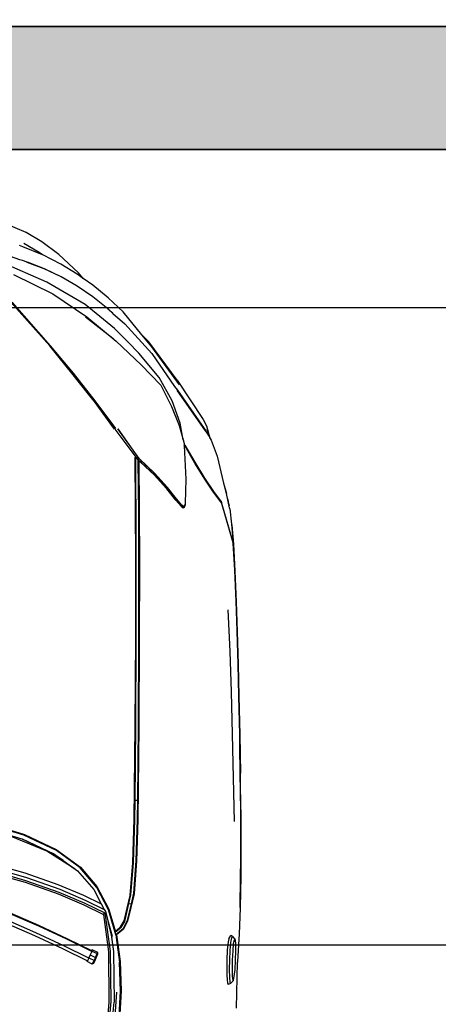
# Model space of a CAD drawing. Units: inches. Extents: x -4737294 to -4736756, y 1716389 to 1717040.
# Tile 15 of 25: x -4737127 to -4737096, y 1716597 to 1716669. Entities that reach past the tile are written whole.
import ezdxf

# ---------------------------------------------------------------- set-up
doc = ezdxf.new("R2010")
doc.units = ezdxf.units.IN
doc.header["$MEASUREMENT"] = 0
for name, color, linetype, lineweight in [('A-ANNO-DIMS', 2, 'Continuous', 18), ('A-EQPM-VEHI', 250, 'Continuous', 13), ('A-WALL-PATT', 244, 'Continuous', 13), ('walls', 252, 'Continuous', 35)]:
    doc.layers.add(name, color=color, linetype=linetype, lineweight=lineweight)
doc.layers.add('Edges', color=250, linetype='Continuous')
doc.styles.get("Standard").update_dxf_attribs({"font": 'arial.ttf'})
doc.dimstyles.get("Standard").update_dxf_attribs({"dimtxt": 8, "dimasz": 0.18, "dimexe": 0.18, "dimexo": 0.0625, "dimgap": 0.09, "dimtad": 0, "dimtih": 1, "dimtoh": 1, "dimzin": 0, "dimdsep": 46, "dimlunit": 3, "dimtxsty": 'Standard', "dimcen": 0.09, "dimadec": 0, "dimazin": 0, "dimtfac": 1, "dimtofl": 0, "dimtmove": 0, "dimatfit": 3, "dimfxl": 1, "dimtolj": 1, "dimtzin": 0, "dimarcsym": 0})

# ---------------------------------------------------------------- blocks, each defined once
blk = doc.blocks.new('Nissan Qashqai pl')
at = {"layer": 'Edges'}
for p, q in [((7.8676, 12.8123), (7.7998, 12.7928)), ((7.8012, 12.7929), (7.8681, 12.8121)), ((7.8107, 12.8065), (7.8363, 12.8097)), ((7.8363, 12.8097), (7.8676, 12.8123)), ((7.8363, 12.8097), (7.8381, 12.81)), ((7.8381, 12.81), (7.87, 12.8126)), ((7.8676, 12.8123), (7.8681, 12.8121)), ((7.869, 12.8124), (7.8681, 12.8121)), ((7.9137, 12.815), (7.869, 12.8124)), ((7.87, 12.8126), (7.9151, 12.8152)), ((7.9658, 12.8172), (7.9137, 12.815)), ((7.9151, 12.8152), (7.9668, 12.8174)), ((8.016, 12.8189), (7.9658, 12.8172)), ((7.9668, 12.8174), (8.0168, 12.8191)), ((8.0713, 12.8205), (8.016, 12.8189)), ((8.0168, 12.8191), (8.0718, 12.8207)), ((8.1249, 12.8218), (8.0713, 12.8205)), ((8.0718, 12.8207), (8.1251, 12.822)), ((8.1176, 12.8087), (8.1888, 12.8107)), ((8.1901, 12.8232), (8.1249, 12.8218)), ((8.1251, 12.822), (8.1902, 12.8233)), ((8.1888, 12.8107), (8.2622, 12.8125)), ((8.2094, 12.8235), (8.1901, 12.8232)), ((8.1902, 12.8233), (8.2543, 12.8243)), ((8.2543, 12.8243), (8.2094, 12.8235)), ((8.2543, 12.8243), (8.2094, 12.8235)), ((8.2544, 12.8242), (8.2094, 12.8235)), ((8.2693, 12.8245), (8.2543, 12.8243)), ((8.3166, 12.8249), (8.2544, 12.8242)), ((8.2622, 12.8125), (8.3356, 12.8141)), ((8.3098, 12.825), (8.2693, 12.8245)), ((8.3159, 12.825), (8.2693, 12.8245)), ((8.3159, 12.825), (8.3098, 12.825)), ((8.3159, 12.825), (8.3163, 12.825)), ((8.3163, 12.825), (8.3657, 12.8252)), ((8.3163, 12.825), (8.3597, 12.8252)), ((8.3764, 12.8251), (8.3166, 12.8249)), ((8.3597, 12.8252), (8.3657, 12.8252)), ((8.3657, 12.8252), (8.3663, 12.8252)), ((8.3663, 12.8252), (8.3747, 12.8252)), ((8.3764, 12.8251), (8.3663, 12.8252)), ((8.3747, 12.8252), (8.3757, 12.8252)), ((8.3757, 12.8252), (8.4282, 12.8249)), ((8.4069, 12.8249), (8.3764, 12.8251)), ((8.4219, 12.8246), (8.4069, 12.8249)), ((8.4292, 12.8248), (8.4069, 12.8249)), ((8.4282, 12.8249), (8.4799, 12.8239)), ((8.4799, 12.8239), (8.4292, 12.8248)), ((8.4799, 12.8239), (8.4811, 12.8239)), ((8.4811, 12.8239), (8.5241, 12.8222)), ((8.5241, 12.8222), (8.5707, 12.8193)), ((8.5287, 12.8112), (8.5269, 12.8082)), ((8.5287, 12.8112), (8.5331, 12.815)), ((8.5287, 12.8112), (8.531, 12.8095)), ((8.5347, 12.8159), (8.5331, 12.815)), ((8.5331, 12.815), (8.5346, 12.8138)), ((8.5346, 12.8138), (8.5406, 12.8125)), ((8.5407, 12.8167), (8.5347, 12.8159)), ((8.5406, 12.8125), (8.5526, 12.8114)), ((8.5527, 12.8169), (8.5407, 12.8167)), ((8.5526, 12.8114), (8.5681, 12.8107)), ((8.5682, 12.8164), (8.5527, 12.8169)), ((8.5681, 12.8107), (8.5836, 12.8104)), ((8.5837, 12.8154), (8.5682, 12.8164)), ((8.5707, 12.8193), (8.5719, 12.8193)), ((8.6489, 12.8179), (8.5719, 12.8193)), ((8.5836, 12.8104), (8.5957, 12.8107)), ((8.5958, 12.8141), (8.5837, 12.8154)), ((8.5957, 12.8107), (8.6017, 12.8114)), ((8.6018, 12.8129), (8.5958, 12.8141)), ((8.6017, 12.8114), (8.6032, 12.8121)), ((8.6032, 12.8121), (8.6018, 12.8129)), ((8.6073, 12.808), (8.6032, 12.8121)), ((7.7223, 12.7851), (7.7673, 12.7961)), ((7.7673, 12.7961), (7.8058, 12.8055)), ((7.7673, 12.7961), (7.7848, 12.8012)), ((7.7835, 12.8007), (7.7835, 12.8007)), ((7.8087, 12.8062), (7.7848, 12.8012)), ((7.7865, 12.8013), (7.7866, 12.8013)), ((7.7936, 12.8029), (7.7977, 12.8038)), ((7.8106, 12.8065), (7.8087, 12.8062)), ((7.8106, 12.8065), (7.8107, 12.8065)), ((7.9803, 12.803), (8.05, 12.8066)), ((8.05, 12.8066), (8.1176, 12.8087)), ((8.5322, 12.8047), (8.5269, 12.8082)), ((8.531, 12.8095), (8.5385, 12.8079)), ((8.5322, 12.8047), (8.5375, 12.8036)), ((8.5375, 12.8036), (8.5513, 12.8023)), ((8.5385, 12.8079), (8.5518, 12.8066)), ((8.5513, 12.8023), (8.5678, 12.8016)), ((8.5518, 12.8066), (8.568, 12.8059)), ((8.5678, 12.8016), (8.5844, 12.8014)), ((8.568, 12.8059), (8.5842, 12.8057)), ((8.5842, 12.8057), (8.5974, 12.8061)), ((8.5844, 12.8014), (8.5921, 12.8016)), ((8.5921, 12.8016), (8.6021, 12.8022)), ((8.5974, 12.8061), (8.6049, 12.8069)), ((8.6021, 12.8022), (8.6065, 12.8027)), ((8.6049, 12.8069), (8.6073, 12.808)), ((8.6065, 12.8027), (8.6093, 12.804)), ((8.6073, 12.808), (8.6093, 12.804)), ((7.6953, 12.7753), (7.7223, 12.7851)), ((7.7591, 12.7641), (7.7814, 12.7791)), ((7.7828, 12.7793), (7.7606, 12.7644)), ((7.7814, 12.7791), (7.7991, 12.7923)), ((7.7984, 12.7909), (7.7828, 12.7793)), ((7.7976, 12.792), (7.7991, 12.7923)), ((7.8007, 12.7926), (7.7984, 12.7909)), ((7.7991, 12.7923), (7.7998, 12.7928)), ((7.7995, 12.7924), (7.8007, 12.7926)), ((7.8012, 12.7929), (7.8007, 12.7926)), ((7.5946, 12.718), (7.6608, 12.7617)), ((7.6113, 12.7186), (7.6759, 12.7633)), ((7.6799, 12.7658), (7.6125, 12.719)), ((7.6608, 12.7617), (7.6712, 12.7675)), ((7.6712, 12.7675), (7.6721, 12.7679)), ((7.6926, 12.7737), (7.6721, 12.7679)), ((7.6759, 12.7633), (7.6793, 12.7657)), ((7.6911, 12.7728), (7.6774, 12.7688)), ((7.6793, 12.7657), (7.6802, 12.766)), ((7.6799, 12.7658), (7.6802, 12.766)), ((7.6802, 12.766), (7.6809, 12.7664)), ((7.6809, 12.7664), (7.6911, 12.7728)), ((7.6911, 12.7728), (7.6926, 12.7737)), ((7.6926, 12.7737), (7.6953, 12.7753)), ((7.7325, 12.7476), (7.7591, 12.7641)), ((7.7606, 12.7644), (7.7341, 12.7478)), ((7.7038, 12.731), (7.7325, 12.7476)), ((7.7341, 12.7478), (7.7056, 12.7314)), ((7.6949, 12.7283), (7.667, 12.723)), ((7.6708, 12.7217), (7.6949, 12.7283)), ((7.6949, 12.7283), (7.701, 12.73)), ((7.701, 12.73), (7.7024, 12.7301)), ((7.7024, 12.7301), (7.7038, 12.731)), ((7.7024, 12.7301), (7.7034, 12.7301)), ((7.7056, 12.7314), (7.7034, 12.7301)), ((7.7034, 12.7301), (7.7048, 12.7302)), ((7.7048, 12.7302), (7.7608, 12.7329)), ((7.7058, 12.7308), (7.7048, 12.7302)), ((7.7608, 12.7329), (7.8014, 12.7318)), ((7.7688, 12.7328), (7.7688, 12.734)), ((7.8014, 12.7318), (7.8022, 12.7316)), ((7.8022, 12.7316), (7.8037, 12.7315)), ((7.8022, 12.7316), (7.8072, 12.73)), ((7.8037, 12.7315), (7.8096, 12.7294)), ((7.8072, 12.73), (7.8045, 12.7263)), ((7.8062, 12.725), (7.8087, 12.7283)), ((7.8096, 12.7294), (7.8066, 12.7254)), ((7.8072, 12.73), (7.8087, 12.7283)), ((7.5946, 12.718), (7.5304, 12.6704)), ((7.6024, 12.7221), (7.5387, 12.6759)), ((7.5501, 12.6757), (7.6051, 12.7139)), ((7.6051, 12.7139), (7.6113, 12.7186)), ((7.6051, 12.7139), (7.6111, 12.7181)), ((7.6118, 12.7186), (7.6111, 12.7181)), ((7.6125, 12.719), (7.6118, 12.7186)), ((7.667, 12.723), (7.6295, 12.7097)), ((7.6386, 12.7089), (7.6708, 12.7217)), ((7.7938, 12.7171), (7.7748, 12.7018)), ((7.7959, 12.7161), (7.7772, 12.7011)), ((7.8045, 12.7263), (7.7938, 12.7171)), ((7.8062, 12.725), (7.7959, 12.7161)), ((7.8066, 12.7254), (7.8062, 12.725)), ((7.6295, 12.7097), (7.59, 12.6877)), ((7.6032, 12.6908), (7.6386, 12.7089)), ((7.7748, 12.7018), (7.7507, 12.6803)), ((7.753, 12.6794), (7.776, 12.6999)), ((7.776, 12.6999), (7.7539, 12.68)), ((7.7772, 12.7011), (7.776, 12.6999)), ((7.59, 12.6877), (7.5492, 12.654)), ((7.5687, 12.6579), (7.6032, 12.6908)), ((7.7261, 12.6543), (7.7507, 12.6803)), ((7.753, 12.6794), (7.7281, 12.6524)), ((7.7507, 12.6803), (7.7286, 12.6561)), ((7.7539, 12.68), (7.7324, 12.6565)), ((7.5501, 12.6757), (7.5001, 12.6302)), ((7.5387, 12.6759), (7.5184, 12.6591)), ((7.5184, 12.6591), (7.5304, 12.6704)), ((7.5184, 12.6591), (7.4801, 12.6274)), ((7.5289, 12.6158), (7.5687, 12.6579)), ((7.5492, 12.654), (7.531, 12.6359)), ((7.7261, 12.6543), (7.6762, 12.6186)), ((7.6762, 12.6186), (7.7233, 12.6514)), ((7.6771, 12.6135), (7.7215, 12.6473)), ((7.7215, 12.6473), (7.7221, 12.6478)), ((7.7232, 12.6486), (7.7221, 12.6478)), ((7.7281, 12.6524), (7.7232, 12.6486)), ((7.7245, 12.6486), (7.7232, 12.6486)), ((7.7267, 12.6539), (7.7233, 12.6514)), ((7.7261, 12.6476), (7.7238, 12.6476)), ((7.7294, 12.6487), (7.7245, 12.6486)), ((7.7279, 12.6477), (7.7261, 12.6476)), ((7.7286, 12.6561), (7.7267, 12.6539)), ((7.8048, 12.6483), (7.7279, 12.6477)), ((7.7299, 12.6537), (7.7281, 12.6524)), ((7.7281, 12.6524), (7.7349, 12.6524)), ((7.731, 12.6487), (7.7294, 12.6487)), ((7.7324, 12.6565), (7.7299, 12.6537)), ((7.7299, 12.6537), (7.7334, 12.6537)), ((7.764, 12.6489), (7.731, 12.6487)), ((7.7334, 12.6537), (7.8083, 12.6544)), ((7.7349, 12.6524), (7.768, 12.6527)), ((7.7662, 12.6489), (7.764, 12.6489)), ((7.7811, 12.649), (7.7662, 12.6489)), ((7.768, 12.6527), (7.7692, 12.6527)), ((7.7692, 12.6527), (7.7844, 12.6528)), ((7.7822, 12.649), (7.7811, 12.649)), ((7.8057, 12.6491), (7.7822, 12.649)), ((7.7844, 12.6528), (7.8078, 12.653)), ((7.9014, 12.6487), (7.8048, 12.6483)), ((7.8233, 12.6492), (7.8057, 12.6491)), ((7.8078, 12.653), (7.8233, 12.6531)), ((7.8083, 12.6544), (7.904, 12.6547)), ((7.8233, 12.6531), (7.9036, 12.6534)), ((7.902, 12.6495), (7.8233, 12.6492)), ((8.0273, 12.6485), (7.9014, 12.6487)), ((8.0275, 12.6493), (7.902, 12.6495)), ((7.9036, 12.6534), (8.0275, 12.6533)), ((7.904, 12.6547), (8.0276, 12.6545)), ((8.1753, 12.6479), (8.0273, 12.6485)), ((8.0275, 12.6533), (8.1755, 12.6527)), ((8.1754, 12.6487), (8.0275, 12.6493)), ((8.0276, 12.6545), (8.1753, 12.6539)), ((8.1753, 12.6539), (8.3324, 12.6521)), ((8.3318, 12.6462), (8.1753, 12.6479)), ((8.3002, 12.6474), (8.1754, 12.6487)), ((8.1755, 12.6527), (8.3005, 12.6514)), ((8.3005, 12.6514), (8.3002, 12.6474)), ((8.332, 12.6471), (8.3002, 12.6474)), ((8.3005, 12.6514), (8.3324, 12.651)), ((8.4049, 12.6437), (8.3318, 12.6462)), ((8.4042, 12.6447), (8.332, 12.6471)), ((8.3324, 12.6521), (8.4022, 12.6498)), ((8.3324, 12.651), (8.4014, 12.6488)), ((8.4014, 12.6488), (8.4559, 12.6451)), ((8.4022, 12.6498), (8.4571, 12.6459)), ((8.4588, 12.6405), (8.4042, 12.6447)), ((8.4559, 12.6451), (8.4736, 12.6409)), ((8.4571, 12.6459), (8.5029, 12.635)), ((7.4827, 12.6103), (7.5001, 12.6302)), ((7.531, 12.6359), (7.5081, 12.6131)), ((7.531, 12.6359), (7.5301, 12.6353)), ((8.4595, 12.6395), (8.4049, 12.6437)), ((8.4729, 12.6372), (8.4588, 12.6405)), ((8.5025, 12.6293), (8.4595, 12.6395)), ((8.4729, 12.6372), (8.4736, 12.6409)), ((8.5032, 12.6301), (8.4729, 12.6372)), ((8.4736, 12.6409), (8.5018, 12.6344)), ((8.5018, 12.6344), (8.5155, 12.6274)), ((8.5125, 12.6231), (8.5025, 12.6293)), ((8.5029, 12.635), (8.5163, 12.6279)), ((8.5132, 12.624), (8.5032, 12.6301)), ((8.5163, 12.6279), (8.5237, 12.6189)), ((7.4801, 12.6274), (7.4565, 12.6023)), ((7.5081, 12.6131), (7.4679, 12.5634)), ((7.4884, 12.5664), (7.5289, 12.6158)), ((7.5243, 12.6101), (7.5286, 12.6146)), ((7.676, 12.6152), (7.6296, 12.5803)), ((7.6769, 12.6129), (7.6306, 12.5791)), ((8.4814, 12.6029), (8.5166, 12.6135)), ((8.5216, 12.6139), (8.4838, 12.6027)), ((8.5177, 12.617), (8.5125, 12.6231)), ((8.5132, 12.624), (8.5216, 12.6139)), ((8.5155, 12.6274), (8.5258, 12.6151)), ((8.5166, 12.6135), (8.5197, 12.6145)), ((8.5197, 12.6145), (8.5177, 12.617)), ((8.5197, 12.6145), (8.5216, 12.6139)), ((8.5258, 12.6151), (8.5216, 12.6139)), ((8.5237, 12.6189), (8.5259, 12.6162)), ((8.5259, 12.6162), (8.5258, 12.6151)), ((8.5258, 12.6151), (8.5304, 12.6157)), ((8.5259, 12.6162), (8.5294, 12.6167)), ((8.5294, 12.6167), (8.5706, 12.6226)), ((8.5304, 12.6157), (8.5715, 12.6215)), ((8.5304, 12.6157), (8.5304, 12.6157)), ((8.5538, 12.6111), (8.6387, 12.6123)), ((8.5706, 12.6226), (8.6197, 12.6241)), ((8.6203, 12.6229), (8.5715, 12.6215)), ((8.6197, 12.6241), (8.6683, 12.6215)), ((8.6203, 12.6229), (8.6204, 12.6229)), ((8.6721, 12.6201), (8.6204, 12.6229)), ((8.622, 12.6161), (8.6699, 12.6132)), ((8.6721, 12.6093), (8.6387, 12.6123)), ((7.4565, 12.6023), (7.4354, 12.5766)), ((7.4542, 12.5765), (7.4744, 12.6015)), ((7.475, 12.6016), (7.4549, 12.5767)), ((7.4744, 12.6015), (7.4804, 12.6079)), ((7.4762, 12.6028), (7.475, 12.6016)), ((7.4752, 12.6016), (7.4762, 12.6028)), ((7.4762, 12.6028), (7.478, 12.6049)), ((7.4804, 12.6079), (7.478, 12.6049)), ((7.478, 12.6049), (7.479, 12.6061)), ((7.479, 12.6061), (7.4815, 12.6089)), ((7.479, 12.6061), (7.4801, 12.6074)), ((7.4801, 12.6074), (7.4804, 12.6079)), ((7.4804, 12.6079), (7.4807, 12.6082)), ((7.4804, 12.6079), (7.4804, 12.6079)), ((7.4807, 12.6082), (7.4821, 12.6097)), ((7.4815, 12.6089), (7.4821, 12.6097)), ((7.4821, 12.6097), (7.4827, 12.6103)), ((7.4882, 12.5645), (7.5243, 12.6101)), ((8.4444, 12.5834), (8.4814, 12.6029)), ((8.4838, 12.6027), (8.4462, 12.5833)), ((8.468, 12.5648), (8.4831, 12.5957)), ((8.4725, 12.563), (8.4889, 12.5969)), ((8.4737, 12.5908), (8.4831, 12.5957)), ((8.4831, 12.5957), (8.4867, 12.5977)), ((8.4867, 12.5977), (8.5039, 12.6023)), ((8.4889, 12.5969), (8.5531, 12.6055)), ((8.4914, 12.5942), (8.4889, 12.5969)), ((8.4914, 12.5942), (8.5544, 12.6026)), ((8.5039, 12.6023), (8.528, 12.6088)), ((8.5216, 12.6068), (8.5039, 12.6023)), ((8.5216, 12.6068), (8.5538, 12.6111)), ((8.5301, 12.609), (8.5216, 12.6068)), ((8.5531, 12.6055), (8.6375, 12.6066)), ((8.5544, 12.6026), (8.6386, 12.6037)), ((8.6375, 12.6066), (8.7481, 12.5968)), ((8.6386, 12.6037), (8.7491, 12.594)), ((7.6296, 12.5803), (7.5827, 12.5441)), ((7.6301, 12.5787), (7.618, 12.5691)), ((7.6306, 12.5791), (7.6301, 12.5787)), ((8.4122, 12.5558), (8.4444, 12.5834)), ((8.4462, 12.5833), (8.4134, 12.5554)), ((8.4499, 12.5782), (8.4737, 12.5908)), ((8.4594, 12.5611), (8.4737, 12.5908)), ((8.4756, 12.5615), (8.4914, 12.5942)), ((8.5554, 12.5847), (8.551, 12.5757)), ((8.5529, 12.5751), (8.5572, 12.5841)), ((8.5574, 12.5849), (8.5554, 12.5847)), ((8.5572, 12.5841), (8.5554, 12.5847)), ((8.5639, 12.581), (8.5572, 12.5841)), ((8.5574, 12.5849), (8.5584, 12.5846)), ((8.5582, 12.5845), (8.5574, 12.5849)), ((8.5584, 12.5846), (8.5649, 12.5816)), ((8.5595, 12.572), (8.5639, 12.581)), ((8.5687, 12.5791), (8.5639, 12.581)), ((8.5644, 12.5701), (8.5687, 12.5791)), ((8.5649, 12.5816), (8.5693, 12.5799)), ((8.5687, 12.5791), (8.5693, 12.5799)), ((8.5749, 12.5757), (8.5687, 12.5791)), ((8.5693, 12.5799), (8.5739, 12.5774)), ((7.4354, 12.5766), (7.4239, 12.5604)), ((7.4679, 12.5634), (7.4302, 12.4993)), ((7.4363, 12.5502), (7.4542, 12.5765)), ((7.4549, 12.5767), (7.4369, 12.5504)), ((7.4498, 12.5093), (7.4884, 12.5664)), ((7.618, 12.5691), (7.5829, 12.5411)), ((7.618, 12.5691), (7.584, 12.5429)), ((8.4183, 12.5508), (8.4499, 12.5782)), ((8.4493, 12.5212), (8.468, 12.5648)), ((8.454, 12.5196), (8.4725, 12.563)), ((8.5527, 12.5749), (8.5323, 12.5332)), ((8.5537, 12.5747), (8.5332, 12.5329)), ((8.5647, 12.57), (8.5441, 12.5279)), ((8.5487, 12.5256), (8.5692, 12.5674)), ((8.5527, 12.5749), (8.551, 12.5757)), ((8.551, 12.5757), (8.5528, 12.5751)), ((8.5528, 12.5751), (8.5527, 12.5749)), ((8.5528, 12.5751), (8.5529, 12.5751)), ((8.5529, 12.5751), (8.5537, 12.5747)), ((8.5537, 12.5747), (8.5595, 12.572)), ((8.5595, 12.572), (8.5644, 12.5701)), ((8.5644, 12.5701), (8.5647, 12.57)), ((8.5647, 12.57), (8.5692, 12.5675)), ((8.5692, 12.5674), (8.5692, 12.5675)), ((8.5692, 12.5675), (8.5705, 12.5668)), ((8.5705, 12.5668), (8.5692, 12.5674)), ((8.5749, 12.5757), (8.5705, 12.5668)), ((8.5739, 12.5774), (8.5749, 12.5757)), ((7.4147, 12.5524), (7.3837, 12.5197)), ((7.4166, 12.5503), (7.3997, 12.5227)), ((7.4239, 12.5604), (7.4147, 12.5524)), ((7.4239, 12.5604), (7.4166, 12.5503)), ((7.4205, 12.5229), (7.4363, 12.5502)), ((7.4369, 12.5504), (7.4211, 12.5232)), ((8.3826, 12.5151), (8.4122, 12.5558)), ((8.4134, 12.5554), (8.3844, 12.5157)), ((8.4154, 12.5468), (8.3852, 12.4994)), ((8.3901, 12.5113), (8.4154, 12.5468)), ((8.4011, 12.5269), (8.4154, 12.5468)), ((8.4156, 12.547), (8.4154, 12.5468)), ((8.4156, 12.547), (8.4183, 12.5508)), ((8.4411, 12.5178), (8.4594, 12.5611)), ((8.4571, 12.5184), (8.4756, 12.5615)), ((7.5827, 12.5441), (7.5369, 12.5057)), ((7.584, 12.5429), (7.5568, 12.5201)), ((7.5829, 12.5411), (7.5568, 12.5201)), ((8.5323, 12.5332), (8.5103, 12.4859)), ((8.5332, 12.5329), (8.5112, 12.4856)), ((7.3837, 12.5197), (7.3624, 12.4907)), ((7.3997, 12.5227), (7.3845, 12.4925)), ((7.4071, 12.4948), (7.4205, 12.5229)), ((7.4211, 12.5232), (7.4078, 12.4951)), ((7.5568, 12.5201), (7.5371, 12.5042)), ((8.3573, 12.4618), (8.3826, 12.5151)), ((8.3844, 12.5157), (8.3582, 12.4606)), ((8.4011, 12.5269), (8.3901, 12.5113)), ((8.3904, 12.512), (8.4011, 12.5269)), ((8.4217, 12.4622), (8.4411, 12.5178)), ((8.4296, 12.4651), (8.4493, 12.5212)), ((8.4343, 12.4637), (8.454, 12.5196)), ((8.4375, 12.4627), (8.4571, 12.5184)), ((8.5441, 12.5279), (8.5222, 12.4807)), ((8.5269, 12.4785), (8.5487, 12.5256)), ((7.4302, 12.4993), (7.3963, 12.4227)), ((7.4172, 12.4431), (7.4498, 12.5093)), ((7.5369, 12.5057), (7.4635, 12.4408)), ((7.4638, 12.439), (7.5371, 12.5042)), ((8.3852, 12.4994), (8.3608, 12.4393)), ((8.3646, 12.4572), (8.39, 12.5111)), ((8.3648, 12.4579), (8.39, 12.5111)), ((8.39, 12.5111), (8.3852, 12.4994)), ((8.39, 12.5111), (8.3901, 12.5113)), ((8.3901, 12.5113), (8.3904, 12.512)), ((7.3624, 12.4907), (7.347, 12.4644)), ((7.3805, 12.4866), (7.3655, 12.4604)), ((7.3843, 12.492), (7.3707, 12.4592)), ((7.3843, 12.492), (7.3805, 12.4866)), ((7.3845, 12.4925), (7.3843, 12.492)), ((7.3962, 12.466), (7.4071, 12.4948)), ((7.4078, 12.4951), (7.3969, 12.4665)), ((8.5103, 12.4859), (8.4895, 12.4381)), ((8.5112, 12.4856), (8.4904, 12.4377)), ((8.5222, 12.4807), (8.5014, 12.4329)), ((7.347, 12.4644), (7.3309, 12.4276)), ((7.3965, 12.4655), (7.3951, 12.462)), ((7.3965, 12.4655), (7.3962, 12.466)), ((7.3969, 12.4665), (7.3965, 12.4655)), ((7.3968, 12.4649), (7.3967, 12.4651)), ((8.4084, 12.3907), (8.4296, 12.4651)), ((8.4133, 12.3896), (8.4343, 12.4637)), ((8.4165, 12.3888), (8.4375, 12.4627)), ((8.5062, 12.431), (8.5269, 12.4785)), ((7.3707, 12.4592), (7.3688, 12.4532)), ((7.3925, 12.4542), (7.3845, 12.4306)), ((7.3938, 12.4583), (7.3925, 12.4542)), ((7.3951, 12.462), (7.3938, 12.4583)), ((8.3296, 12.3703), (8.3573, 12.4618)), ((8.3582, 12.4606), (8.3311, 12.3708)), ((8.3377, 12.3689), (8.3646, 12.4572)), ((8.3646, 12.4572), (8.3648, 12.4579)), ((8.3648, 12.4579), (8.3648, 12.4579)), ((8.4009, 12.3883), (8.4217, 12.4622))]:
    blk.add_line(p, q, dxfattribs=at)
blk = doc.blocks.new('car')
blk.add_blockref('Nissan Qashqai pl', (-9.7433, -11.9151))
blk = doc.blocks.new('*D63')
at = {"layer": 'A-ANNO-DIMS', "color": 0, "lineweight": -2, "transparency": 16777216}
for p, q in [((-4737062.207, 1716647.493), (-4737270.324, 1716647.493)), ((-4737270.144, 1716647.313), (-4737270.144, 1716628.418)), ((-4737270.144, 1716601.064), (-4737270.144, 1716619.959)), ((-4737062.207, 1716600.884), (-4737270.324, 1716600.884))]:
    blk.add_line(p, q, dxfattribs=at)
at = {"layer": 'A-ANNO-DIMS', "color": 0, "transparency": 16777216}
for points in [[(-4737270.174, 1716647.313), (-4737270.114, 1716647.313), (-4737270.144, 1716647.493)], [(-4737270.174, 1716601.064), (-4737270.114, 1716601.064), (-4737270.144, 1716600.884)]]:
    blk.add_solid(points, dxfattribs=at)
at = {"layer": 'Defpoints', "color": 0, "transparency": 16777216}
for p in [(-4737270.144, 1716647.493), (-4737062.144, 1716647.493), (-4737062.144, 1716600.884)]:
    blk.add_point(p, dxfattribs=at)
at = {"layer": 'A-ANNO-DIMS', "color": 0, "transparency": 16777216, "insert": (-4737270.144, 1716624.188), "char_height": 8, "attachment_point": 5}
blk.add_mtext('\\A1;3\'-10 1/2"', dxfattribs=at)

msp = doc.modelspace()

# ---------------------------------------------------------------- hatches: boundary and pattern name
at = {"layer": 'A-WALL-PATT'}
h = msp.add_hatch(color=256, dxfattribs=at)
h.dxf.hatch_style = 1
h.paths.add_polyline_path([(-4737206.144, 1716844.565), (-4737110.144, 1716844.565), (-4737110.144, 1716823.907), (-4737105.644, 1716823.907), (-4737105.644, 1716844.565), (-4737098.44, 1716844.565), (-4737098.44, 1716849.065), (-4737206.144, 1716849.065), (-4737206.144, 1716993.065), (-4736864.144, 1716993.065), (-4736864.144, 1716849.065), (-4736963.275, 1716849.065), (-4736994.446, 1716849.065), (-4736997.144, 1716849.065), (-4736997.144, 1716844.565), (-4736864.144, 1716844.565), (-4736864.144, 1716668.565), (-4736934.391, 1716668.565), (-4736934.391, 1716664.065), (-4736864.144, 1716664.065), (-4736864.144, 1716462.065), (-4736855.144, 1716462.065), (-4736855.144, 1717002.065), (-4737215.144, 1717002.065), (-4737215.144, 1716462.065), (-4737206.144, 1716462.065), (-4737206.144, 1716659.065), (-4737062.144, 1716659.065), (-4737062.144, 1716647.493), (-4737057.644, 1716647.493), (-4737057.644, 1716796.565), (-4737071.812, 1716796.565), (-4737071.812, 1716792.065), (-4737070.805, 1716792.065), (-4737062.144, 1716792.065), (-4737062.144, 1716668.065), (-4737206.144, 1716668.065), (-4737206.144, 1716792.065), (-4737093.784, 1716792.065), (-4737093.784, 1716796.565), (-4737206.144, 1716796.565)])

# ---------------------------------------------------------------- linework, layer by layer
at = {"layer": 'walls'}
for p, q in [((-4737206.144, 1716668.065), (-4737062.144, 1716668.065)), ((-4737206.144, 1716659.065), (-4737062.144, 1716659.065))]:
    msp.add_line(p, q, dxfattribs=at)

# ---------------------------------------------------------------- block references
at = {"layer": 'A-EQPM-VEHI', "xscale": 43.56002006885659, "yscale": 43.56002006885659, "zscale": 43.56002006885659, "rotation": 270}
msp.add_blockref('car', (-4737150.017, 1716548.61), dxfattribs=at)

# ---------------------------------------------------------------- dimensions: what is measured, and where the dimension line sits
at = {"layer": 'A-ANNO-DIMS'}
dim = msp.add_linear_dim(base=(-4737270.144, 1716647.493), p1=(-4737062.144, 1716600.884), p2=(-4737062.144, 1716647.493), angle=90, dimstyle='Standard', override={"dimdec": 1, "dimlfac": 1, "dimrnd": 0, "dimzin": 1, "dimdsep": 46, "dimlunit": 4, "dimfrac": 2}, dxfattribs=at)
dim.commit()
dim.dimension.update_dxf_attribs({"geometry": '*D63', "text_midpoint": (-4737270.144, 1716624.188)})

doc.saveas('drawing.dxf')
